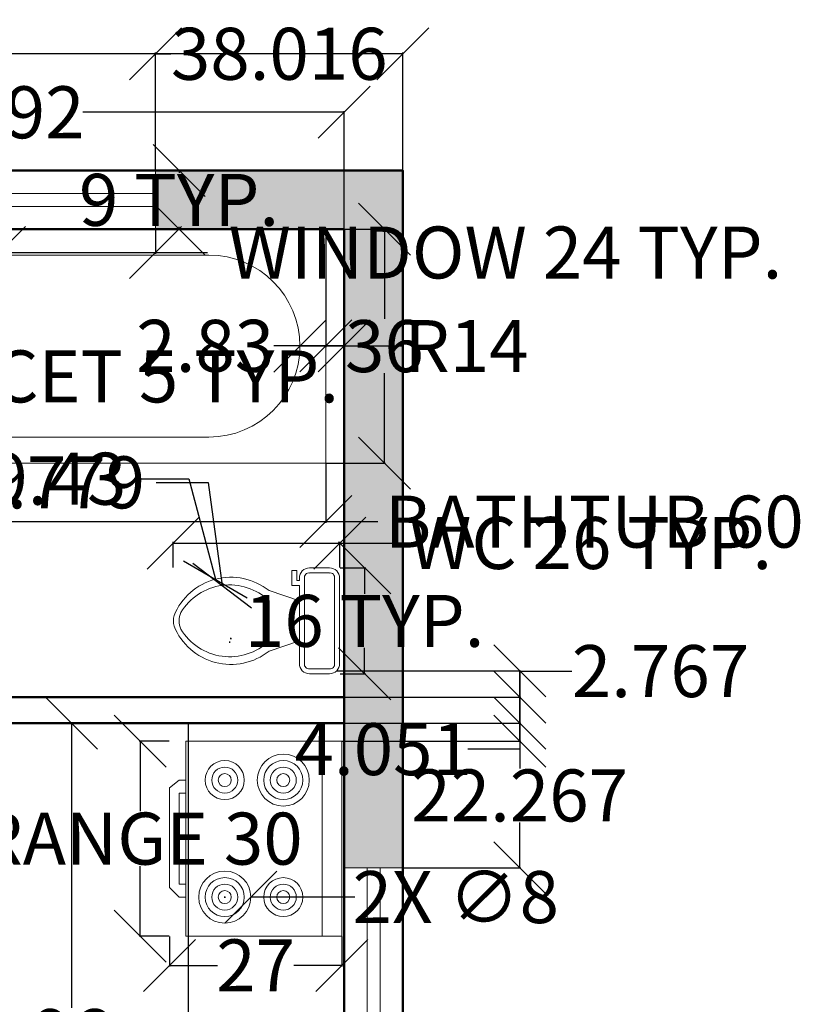
# Model space of a CAD drawing. Units: inches. Extents: x -87 to 308, y -349 to 42.
# Tile 6 of 6: x 188 to 308, y -110 to 42. Entities that reach past the tile are written whole.
import ezdxf

# ---------------------------------------------------------------- set-up
doc = ezdxf.new("R2010")
doc.units = ezdxf.units.IN
doc.header["$MEASUREMENT"] = 0
for name, color, linetype, lineweight in [('A-ANNO-DIMS', 2, 'Continuous', 18), ('A-EQPM', 8, 'Continuous', 20), ('A-FLOR-CASE', 9, 'Continuous', 25), ('A-FLOR-FIXT', 9, 'Continuous', 18), ('A-GLAZ', 4, 'Continuous', 18), ('A-WALL', 7, 'Continuous', 50), ('A-WALL-PATT', 251, 'Continuous', 13)]:
    doc.layers.add(name, color=color, linetype=linetype, lineweight=lineweight)
doc.styles.get("Standard").update_dxf_attribs({"font": 'arial.ttf'})
doc.dimstyles.get("Standard").update_dxf_attribs({"dimtxt": 8, "dimasz": 8, "dimexe": 0.18, "dimexo": 0.0625, "dimgap": 0.09, "dimtad": 0, "dimtih": 1, "dimtoh": 1, "dimdec": 0, "dimzin": 0, "dimdsep": 46, "dimlunit": 4, "dimtxsty": 'Standard', "dimblk": 'OBLIQUE', "dimcen": 0.09, "dimadec": 0, "dimazin": 0, "dimtfac": 1, "dimtdec": 0, "dimtofl": 0, "dimtmove": 0, "dimatfit": 3, "dimldrblk": 'OBLIQUE', "dimfxl": 1, "dimtolj": 1, "dimtzin": 0, "dimarcsym": 0})

# ---------------------------------------------------------------- blocks, each defined once
blk = doc.blocks.new('Toilet - top')
for p, q in [((9.5, -6), (9.5, -2)), ((-10, -8.5), (-8, -8.5)), ((-10, -9.5), (-10, -8.5)), ((-7, -9.5), (-10, -9.5)), ((-8, -8.5), (-8, -8)), ((-7, -8), (-7, -9.5)), ((-4, -8), (-6, -14)), ((4, -8), (6, -14)), ((4, -14), (-4, -14))]:
    blk.add_line(p, q)
blk.add_lwpolyline([(-7, -8), (8.5, -8, 0.414214), (10.5, -6), (10.5, -2, 0.414214), (8.5, 0), (-8.5, 0, 0.414214), (-10.5, -2), (-10.5, -6, 0.414214), (-8.5, -8), (-8, -8)], format="xyb")
for points in [[(8.5, -1), (-8.5, -1)], [(-9.5, -2), (-9.5, -6)], [(-8.5, -7), (8.5, -7)]]:
    blk.add_lwpolyline(points)
for centre, radius, start, end in [((-8.62, -1.88), 0.884, 81.8699, 188.1301), ((8.62, -1.88), 0.884, 351.8699, 98.1301), ((-8.62, -6.12), 0.884, 171.8699, 278.1301), ((8.62, -6.12), 0.884, 261.8699, 8.1301), ((3.52, -21.58), 12.17, 141.4691, 247.9714), ((4.2, -21.82), 11.33, 136.3677, 238.9468), ((-3.52, -21.58), 12.17, 292.0284, 38.5307), ((-4.2, -21.82), 11.33, 301.053, 43.6321), ((0, -27.88), 4, 245.7318, 294.2682), ((0, -29), 4, 254.8605, 285.1395)]:
    blk.add_arc(centre, radius, start, end)
blk = doc.blocks.new('Range-Oven - 30 in top')
for p, q in [((0, -3), (30, -3)), ((6, -24), (6, -25)), ((8, -25), (8, -24)), ((8, -24), (22, -24)), ((22, -25), (22, -24)), ((24, -24), (24, -25)), ((6, -25), (7.2, -26.5)), ((24, -25), (22.5, -26.5))]:
    blk.add_line(p, q)
for points in [[(8, -24), (0, -24), (0, 0), (30, 0), (30, -24), (22, -24)], [(8, -25), (22, -25)], [(22.5, -26.5), (7.2, -26.5)]]:
    blk.add_lwpolyline(points)
for centre, radius in [((6, -9), 4), ((6, -9), 3), ((24, -9), 3), ((6, -9), 2), ((24, -9), 2), ((6, -9), 1), ((24, -9), 1), ((6, -18), 3), ((24, -18), 4), ((24, -18), 3), ((6, -18), 2), ((24, -18), 2), ((6, -18), 1), ((24, -18), 1)]:
    blk.add_circle(centre, radius)
blk = doc.blocks.new('Bath Tub - 26 x 60 in.')
for p, q in [((8, -18), (10, -18)), ((9, -17), (9, -19))]:
    blk.add_line(p, q)
blk.add_lwpolyline([(0, -36), (0, 0), (60, 0), (60, -36)], close=True)
for points in [[(6, -4), (42, -4)], [(4, -30), (4, -6)], [(42, -32), (6, -32)]]:
    blk.add_lwpolyline(points)
for radius in [1.5, 1]:
    blk.add_circle((9, -18), radius)
for centre, radius, start, end in [((5.75, -5.75), 1.77, 81.8699, 188.1301), ((42, -18), 14, 270, 90), ((5.75, -30.25), 1.77, 171.8699, 278.1301)]:
    blk.add_arc(centre, radius, start, end)
blk = doc.blocks.new('WIN-48IN')
for p, q in [((0, 5.5), (48, 5.5)), ((0, 3.5), (48, 3.5))]:
    blk.add_line(p, q)
for points in [[(0, 0), (0, 9)], [(48, 9), (48, 0)]]:
    blk.add_lwpolyline(points)
blk = doc.blocks.new('WIN-24IN')
for p, q in [((0, 5.5), (24, 5.5)), ((0, 3.5), (24, 3.5))]:
    blk.add_line(p, q)
for points in [[(0, 0), (0, 9)], [(24, 9), (24, 0)]]:
    blk.add_lwpolyline(points)
blk = doc.blocks.new('_Oblique')
at = {"color": 0, "linetype": 'ByBlock', "lineweight": -2}
blk.add_line((-0.5, -0.5), (0.5, 0.5), dxfattribs=at)
blk = doc.blocks.new('*D25')
at = {"layer": 'A-ANNO-DIMS', "color": 0, "lineweight": -2, "transparency": 16777216}
for p, q in [((184.75, 9.27), (184.75, 5.55)), ((208.75, 9.27), (208.75, 5.55)), ((184.75, 5.73), (208.75, 5.73)), ((208.75, 5.73), (216.75, 5.73))]:
    blk.add_line(p, q, dxfattribs=at)
at = {"layer": 'Defpoints', "color": 0, "transparency": 16777216}
for p in [(184.75, 9.33), (208.75, 9.33), (208.75, 5.73)]:
    blk.add_point(p, dxfattribs=at)
at = {"layer": 'A-ANNO-DIMS', "color": 0, "lineweight": -2, "transparency": 16777216, "xscale": 8, "yscale": 8, "zscale": 8, "rotation": 180}
blk.add_blockref('_Oblique', (184.75, 5.73), dxfattribs=at)
at = {"layer": 'A-ANNO-DIMS', "color": 0, "lineweight": -2, "transparency": 16777216, "xscale": 8, "yscale": 8, "zscale": 8}
blk.add_blockref('_Oblique', (208.75, 5.73), dxfattribs=at)
at = {"layer": 'A-ANNO-DIMS', "color": 0, "transparency": 16777216, "insert": (262.54, 5.73), "char_height": 8, "attachment_point": 5}
blk.add_mtext('\\A1;WINDOW 24 TYP.', dxfattribs=at)
blk = doc.blocks.new('*D26')
at = {"layer": 'A-ANNO-DIMS', "color": 0, "lineweight": -2, "transparency": 16777216}
for p, q in [((208.81, 18.33), (212.53, 18.33)), ((212.35, 18.33), (212.35, 18.01)), ((208.81, 9.33), (212.53, 9.33)), ((212.35, 9.33), (212.35, 9.66))]:
    blk.add_line(p, q, dxfattribs=at)
at = {"layer": 'Defpoints', "color": 0, "transparency": 16777216}
for p in [(208.75, 18.33), (212.35, 18.33), (208.75, 9.33)]:
    blk.add_point(p, dxfattribs=at)
at = {"layer": 'A-ANNO-DIMS', "color": 0, "lineweight": -2, "transparency": 16777216, "xscale": 8, "yscale": 8, "zscale": 8}
for p, rotation in [((212.35, 18.33), 90), ((212.35, 9.33), 270)]:
    blk.add_blockref('_Oblique', p, dxfattribs=dict(at, rotation=rotation))
at = {"layer": 'A-ANNO-DIMS', "color": 0, "transparency": 16777216, "insert": (212.35, 13.83), "char_height": 8, "attachment_point": 5}
blk.add_mtext('\\A1;9 TYP.', dxfattribs=at)
blk = doc.blocks.new('*D27')
at = {"layer": 'A-ANNO-DIMS', "color": 0, "lineweight": -2, "transparency": 16777216}
for p, q in [((211.44, -42.74), (211.44, -38.78)), ((211.44, -38.96), (237.05, -38.96)), ((237.05, -42.74), (237.05, -38.78)), ((237.05, -38.96), (245.05, -38.96))]:
    blk.add_line(p, q, dxfattribs=at)
at = {"layer": 'Defpoints', "color": 0, "transparency": 16777216}
for p in [(237.05, -38.96), (211.44, -42.8), (237.05, -42.8)]:
    blk.add_point(p, dxfattribs=at)
at = {"layer": 'A-ANNO-DIMS', "color": 0, "lineweight": -2, "transparency": 16777216, "xscale": 8, "yscale": 8, "zscale": 8, "rotation": 180}
blk.add_blockref('_Oblique', (211.44, -38.96), dxfattribs=at)
at = {"layer": 'A-ANNO-DIMS', "color": 0, "lineweight": -2, "transparency": 16777216, "xscale": 8, "yscale": 8, "zscale": 8}
blk.add_blockref('_Oblique', (237.05, -38.96), dxfattribs=at)
at = {"layer": 'A-ANNO-DIMS', "color": 0, "transparency": 16777216, "insert": (275.63, -38.96), "char_height": 8, "attachment_point": 5}
blk.add_mtext('\\A1;WC 26 TYP.', dxfattribs=at)
blk = doc.blocks.new('*D28')
at = {"layer": 'A-ANNO-DIMS', "color": 0, "lineweight": -2, "transparency": 16777216}
for p, q in [((237.11, -42.8), (241.07, -42.8)), ((240.89, -42.8), (240.89, -46.76)), ((240.89, -59.07), (240.89, -55.11)), ((237.11, -59.07), (241.07, -59.07))]:
    blk.add_line(p, q, dxfattribs=at)
at = {"layer": 'Defpoints', "color": 0, "transparency": 16777216}
for p in [(237.05, -42.8), (237.05, -59.07), (240.89, -59.07)]:
    blk.add_point(p, dxfattribs=at)
at = {"layer": 'A-ANNO-DIMS', "color": 0, "lineweight": -2, "transparency": 16777216, "xscale": 8, "yscale": 8, "zscale": 8}
for p, rotation in [((240.89, -42.8), 90), ((240.89, -59.07), 270)]:
    blk.add_blockref('_Oblique', p, dxfattribs=dict(at, rotation=rotation))
at = {"layer": 'A-ANNO-DIMS', "color": 0, "transparency": 16777216, "insert": (240.89, -50.94), "char_height": 8, "attachment_point": 5}
blk.add_mtext('\\A1;16 TYP.', dxfattribs=at)
blk = doc.blocks.new('*D31')
at = {"layer": 'A-ANNO-DIMS', "color": 0, "lineweight": -2, "transparency": 16777216}
for p, q in [((151.98, -21.33), (151.98, -13.33)), ((151.98, -13.33), (159.98, -13.33)), ((151.29, -21.33), (152.16, -21.33)), ((151.98, -26.36), (151.98, -21.33)), ((151.29, -26.36), (152.16, -26.36))]:
    blk.add_line(p, q, dxfattribs=at)
at = {"layer": 'Defpoints', "color": 0, "transparency": 16777216}
for p in [(151.23, -21.33), (151.98, -21.33), (151.23, -26.36)]:
    blk.add_point(p, dxfattribs=at)
at = {"layer": 'A-ANNO-DIMS', "color": 0, "lineweight": -2, "transparency": 16777216, "xscale": 8, "yscale": 8, "zscale": 8}
for p, rotation in [((151.98, -21.33), 90), ((151.98, -26.36), 270)]:
    blk.add_blockref('_Oblique', p, dxfattribs=dict(at, rotation=rotation))
at = {"layer": 'A-ANNO-DIMS', "color": 0, "transparency": 16777216, "insert": (200.11, -13.33), "char_height": 8, "attachment_point": 5}
blk.add_mtext('\\A1;FAUCET 5 TYP.', dxfattribs=at)
blk = doc.blocks.new('*D41')
at = {"layer": 'A-ANNO-DIMS', "color": 0, "lineweight": -2, "transparency": 16777216}
for p, q in [((210.82, -69.44), (206.2, -69.44)), ((206.38, -69.44), (206.38, -80.21)), ((206.38, -99.44), (206.38, -88.66)), ((210.82, -99.44), (206.2, -99.44))]:
    blk.add_line(p, q, dxfattribs=at)
at = {"layer": 'Defpoints', "color": 0, "transparency": 16777216}
for p in [(210.88, -69.44), (206.38, -99.44), (210.88, -99.44)]:
    blk.add_point(p, dxfattribs=at)
at = {"layer": 'A-ANNO-DIMS', "color": 0, "lineweight": -2, "transparency": 16777216, "xscale": 8, "yscale": 8, "zscale": 8}
for p, rotation in [((206.38, -69.44), 90), ((206.38, -99.44), 270)]:
    blk.add_blockref('_Oblique', p, dxfattribs=dict(at, rotation=rotation))
at = {"layer": 'A-ANNO-DIMS', "color": 0, "transparency": 16777216, "insert": (206.38, -84.44), "char_height": 8, "attachment_point": 5}
blk.add_mtext('\\A1;RANGE 30', dxfattribs=at)
blk = doc.blocks.new('*D42')
at = {"layer": 'A-ANNO-DIMS', "color": 0, "lineweight": -2, "transparency": 16777216}
for p, q in [((210.88, -99.5), (210.88, -104.12)), ((237.38, -99.5), (237.38, -104.12)), ((210.88, -103.94), (218.24, -103.94)), ((237.38, -103.94), (230.02, -103.94))]:
    blk.add_line(p, q, dxfattribs=at)
at = {"layer": 'Defpoints', "color": 0, "transparency": 16777216}
for p in [(210.88, -99.44), (237.38, -99.44), (237.38, -103.94)]:
    blk.add_point(p, dxfattribs=at)
at = {"layer": 'A-ANNO-DIMS', "color": 0, "lineweight": -2, "transparency": 16777216, "xscale": 8, "yscale": 8, "zscale": 8, "rotation": 180}
blk.add_blockref('_Oblique', (210.88, -103.94), dxfattribs=at)
at = {"layer": 'A-ANNO-DIMS', "color": 0, "lineweight": -2, "transparency": 16777216, "xscale": 8, "yscale": 8, "zscale": 8}
blk.add_blockref('_Oblique', (237.38, -103.94), dxfattribs=at)
at = {"layer": 'A-ANNO-DIMS', "color": 0, "transparency": 16777216, "insert": (224.13, -103.94), "char_height": 8, "attachment_point": 5}
blk.add_mtext('\\A1;27', dxfattribs=at)
blk = doc.blocks.new('*D45')
at = {"layer": 'A-ANNO-DIMS', "color": 0, "lineweight": -2, "transparency": 16777216}
for p, q in [((174.93, -26.73), (174.93, -35.85)), ((234.93, -26.73), (234.93, -35.85)), ((174.93, -35.67), (234.93, -35.67)), ((234.93, -35.67), (242.93, -35.67))]:
    blk.add_line(p, q, dxfattribs=at)
at = {"layer": 'Defpoints', "color": 0, "transparency": 16777216}
for p in [(174.93, -26.67), (234.93, -26.67), (234.93, -35.67)]:
    blk.add_point(p, dxfattribs=at)
at = {"layer": 'A-ANNO-DIMS', "color": 0, "lineweight": -2, "transparency": 16777216, "xscale": 8, "yscale": 8, "zscale": 8, "rotation": 180}
blk.add_blockref('_Oblique', (174.93, -35.67), dxfattribs=at)
at = {"layer": 'A-ANNO-DIMS', "color": 0, "lineweight": -2, "transparency": 16777216, "xscale": 8, "yscale": 8, "zscale": 8}
blk.add_blockref('_Oblique', (234.93, -35.67), dxfattribs=at)
at = {"layer": 'A-ANNO-DIMS', "color": 0, "transparency": 16777216, "insert": (276.19, -35.67), "char_height": 8, "attachment_point": 5}
blk.add_mtext('\\A1;BATHTUB 60', dxfattribs=at)
blk = doc.blocks.new('*D46')
at = {"layer": 'A-ANNO-DIMS', "color": 0, "lineweight": -2, "transparency": 16777216}
for p, q in [((234.99, 9.33), (244.11, 9.33)), ((243.93, 9.33), (243.93, -4.49)), ((243.93, -26.67), (243.93, -12.85)), ((234.99, -26.67), (244.11, -26.67))]:
    blk.add_line(p, q, dxfattribs=at)
at = {"layer": 'Defpoints', "color": 0, "transparency": 16777216}
for p in [(234.93, 9.33), (243.93, 9.33), (234.93, -26.67)]:
    blk.add_point(p, dxfattribs=at)
at = {"layer": 'A-ANNO-DIMS', "color": 0, "lineweight": -2, "transparency": 16777216, "xscale": 8, "yscale": 8, "zscale": 8}
for p, rotation in [((243.93, 9.33), 90), ((243.93, -26.67), 270)]:
    blk.add_blockref('_Oblique', p, dxfattribs=dict(at, rotation=rotation))
at = {"layer": 'A-ANNO-DIMS', "color": 0, "transparency": 16777216, "insert": (243.93, -8.67), "char_height": 8, "attachment_point": 5}
blk.add_mtext('\\A1;36', dxfattribs=at)
blk = doc.blocks.new('*D47')
at = {"layer": 'A-ANNO-DIMS', "color": 0, "lineweight": -2, "transparency": 16777216}
for p, q in [((12.76, 18.39), (12.76, 36.48)), ((246.76, 18.39), (246.76, 36.48)), ((12.76, 36.3), (120.78, 36.3)), ((246.76, 36.3), (138.74, 36.3))]:
    blk.add_line(p, q, dxfattribs=at)
at = {"layer": 'Defpoints', "color": 0, "transparency": 16777216}
for p in [(246.76, 36.3), (12.76, 18.33), (246.76, 18.33)]:
    blk.add_point(p, dxfattribs=at)
at = {"layer": 'A-ANNO-DIMS', "color": 0, "lineweight": -2, "transparency": 16777216, "xscale": 8, "yscale": 8, "zscale": 8, "rotation": 180}
blk.add_blockref('_Oblique', (12.76, 36.3), dxfattribs=at)
at = {"layer": 'A-ANNO-DIMS', "color": 0, "lineweight": -2, "transparency": 16777216, "xscale": 8, "yscale": 8, "zscale": 8}
blk.add_blockref('_Oblique', (246.76, 36.3), dxfattribs=at)
at = {"layer": 'A-ANNO-DIMS', "color": 0, "transparency": 16777216, "insert": (129.76, 36.3), "char_height": 8, "attachment_point": 5}
blk.add_mtext('\\A1;234', dxfattribs=at)
blk = doc.blocks.new('*D50')
at = {"layer": 'A-ANNO-DIMS', "color": 0, "lineweight": -2, "transparency": 16777216}
for p, q in [((208.75, 18.39), (208.75, 36.48)), ((246.76, 18.39), (246.76, 36.48)), ((208.75, 36.3), (211.07, 36.3)), ((246.76, 36.3), (244.45, 36.3))]:
    blk.add_line(p, q, dxfattribs=at)
at = {"layer": 'Defpoints', "color": 0, "transparency": 16777216}
for p in [(246.76, 36.3), (208.75, 18.33), (246.76, 18.33)]:
    blk.add_point(p, dxfattribs=at)
at = {"layer": 'A-ANNO-DIMS', "color": 0, "lineweight": -2, "transparency": 16777216, "xscale": 8, "yscale": 8, "zscale": 8, "rotation": 180}
blk.add_blockref('_Oblique', (208.75, 36.3), dxfattribs=at)
at = {"layer": 'A-ANNO-DIMS', "color": 0, "lineweight": -2, "transparency": 16777216, "xscale": 8, "yscale": 8, "zscale": 8}
blk.add_blockref('_Oblique', (246.76, 36.3), dxfattribs=at)
at = {"layer": 'A-ANNO-DIMS', "color": 0, "transparency": 16777216, "insert": (227.76, 36.3), "char_height": 8, "attachment_point": 5}
blk.add_mtext('\\A1;38.016', dxfattribs=at)
blk = doc.blocks.new('*D57')
at = {"layer": 'A-ANNO-DIMS', "color": 0, "lineweight": -2, "transparency": 16777216}
for p, q in [((237.83, -66.67), (264.91, -66.67)), ((264.73, -66.67), (264.73, -73.63)), ((264.73, -88.94), (264.73, -81.98)), ((246.83, -88.94), (264.91, -88.94))]:
    blk.add_line(p, q, dxfattribs=at)
at = {"layer": 'Defpoints', "color": 0, "transparency": 16777216}
for p in [(237.76, -66.67), (246.76, -88.94), (264.73, -88.94)]:
    blk.add_point(p, dxfattribs=at)
at = {"layer": 'A-ANNO-DIMS', "color": 0, "lineweight": -2, "transparency": 16777216, "xscale": 8, "yscale": 8, "zscale": 8}
for p, rotation in [((264.73, -66.67), 90), ((264.73, -88.94), 270)]:
    blk.add_blockref('_Oblique', p, dxfattribs=dict(at, rotation=rotation))
at = {"layer": 'A-ANNO-DIMS', "color": 0, "transparency": 16777216, "insert": (264.73, -77.8), "char_height": 8, "attachment_point": 5}
blk.add_mtext('\\A1;22.267', dxfattribs=at)
blk = doc.blocks.new('*D61')
at = {"layer": 'A-ANNO-DIMS', "color": 0, "lineweight": -2, "transparency": 16777216}
for p, q in [((145.76, 9.39), (145.76, 27.48)), ((145.76, 27.3), (185.98, 27.3)), ((237.76, 27.3), (197.54, 27.3)), ((237.76, 9.39), (237.76, 27.48))]:
    blk.add_line(p, q, dxfattribs=at)
at = {"layer": 'Defpoints', "color": 0, "transparency": 16777216}
for p in [(237.76, 27.3), (145.76, 9.33), (237.76, 9.33)]:
    blk.add_point(p, dxfattribs=at)
at = {"layer": 'A-ANNO-DIMS', "color": 0, "lineweight": -2, "transparency": 16777216, "xscale": 8, "yscale": 8, "zscale": 8, "rotation": 180}
blk.add_blockref('_Oblique', (145.76, 27.3), dxfattribs=at)
at = {"layer": 'A-ANNO-DIMS', "color": 0, "lineweight": -2, "transparency": 16777216, "xscale": 8, "yscale": 8, "zscale": 8}
blk.add_blockref('_Oblique', (237.76, 27.3), dxfattribs=at)
at = {"layer": 'A-ANNO-DIMS', "color": 0, "transparency": 16777216, "insert": (191.76, 27.3), "char_height": 8, "attachment_point": 5}
blk.add_mtext('\\A1;92', dxfattribs=at)
blk = doc.blocks.new('*D74')
at = {"layer": 'A-ANNO-DIMS', "color": 0, "lineweight": -2, "transparency": 16777216}
for p, q in [((213.7, -66.67), (195.62, -66.67)), ((195.8, -66.67), (195.8, -110.49)), ((195.8, -162.67), (195.8, -118.84)), ((213.7, -162.67), (195.62, -162.67))]:
    blk.add_line(p, q, dxfattribs=at)
at = {"layer": 'Defpoints', "color": 0, "transparency": 16777216}
for p in [(195.8, -66.67), (213.76, -66.67), (213.76, -162.67)]:
    blk.add_point(p, dxfattribs=at)
at = {"layer": 'A-ANNO-DIMS', "color": 0, "lineweight": -2, "transparency": 16777216, "xscale": 8, "yscale": 8, "zscale": 8}
for p, rotation in [((195.8, -66.67), 90), ((195.8, -162.67), 270)]:
    blk.add_blockref('_Oblique', p, dxfattribs=dict(at, rotation=rotation))
at = {"layer": 'A-ANNO-DIMS', "color": 0, "transparency": 16777216, "insert": (195.8, -114.67), "char_height": 8, "attachment_point": 5}
blk.add_mtext('\\A1;96', dxfattribs=at)
blk = doc.blocks.new('*D85')
at = {"layer": 'A-ANNO-DIMS', "color": 0, "lineweight": -2, "transparency": 16777216}
for p, q in [((234.93, 9.27), (234.93, -8.81)), ((237.76, 9.27), (237.76, -8.81)), ((234.93, -8.63), (226.93, -8.63)), ((237.76, -8.63), (234.93, -8.63))]:
    blk.add_line(p, q, dxfattribs=at)
at = {"layer": 'Defpoints', "color": 0, "transparency": 16777216}
for p in [(234.93, 9.33), (237.76, 9.33), (234.93, -8.63)]:
    blk.add_point(p, dxfattribs=at)
at = {"layer": 'A-ANNO-DIMS', "color": 0, "lineweight": -2, "transparency": 16777216, "xscale": 8, "yscale": 8, "zscale": 8}
for p, rotation in [((234.93, -8.63), 179.9999999999999), ((237.76, -8.63), 359.9999999999999)]:
    blk.add_blockref('_Oblique', p, dxfattribs=dict(at, rotation=rotation))
at = {"layer": 'A-ANNO-DIMS', "color": 0, "transparency": 16777216, "insert": (216.38, -8.63), "char_height": 8, "attachment_point": 5}
blk.add_mtext('\\A1;2.83', dxfattribs=at)
blk = doc.blocks.new('*D87')
at = {"layer": 'A-ANNO-DIMS', "color": 0, "lineweight": -2, "transparency": 16777216}
for p, q in [((236.65, -58.62), (264.91, -58.62)), ((264.73, -58.62), (264.73, -62.67)), ((237.83, -62.67), (264.91, -62.67)), ((264.73, -62.67), (264.73, -70.67)), ((264.73, -70.67), (256.73, -70.67))]:
    blk.add_line(p, q, dxfattribs=at)
at = {"layer": 'Defpoints', "color": 0, "transparency": 16777216}
for p in [(236.59, -58.62), (237.76, -62.67), (264.73, -62.67)]:
    blk.add_point(p, dxfattribs=at)
at = {"layer": 'A-ANNO-DIMS', "color": 0, "lineweight": -2, "transparency": 16777216, "xscale": 8, "yscale": 8, "zscale": 8}
for p, rotation in [((264.73, -58.62), 90), ((264.73, -62.67), 270)]:
    blk.add_blockref('_Oblique', p, dxfattribs=dict(at, rotation=rotation))
at = {"layer": 'A-ANNO-DIMS', "color": 0, "transparency": 16777216, "insert": (243.75, -70.67), "char_height": 8, "attachment_point": 5}
blk.add_mtext('\\A1;4.051', dxfattribs=at)
blk = doc.blocks.new('*D88')
at = {"layer": 'A-ANNO-DIMS', "color": 0, "lineweight": -2, "transparency": 16777216}
for p, q in [((264.73, -66.67), (264.73, -58.67)), ((264.73, -58.67), (272.73, -58.67)), ((237.83, -66.67), (264.91, -66.67)), ((264.73, -69.44), (264.73, -66.67)), ((237.44, -69.44), (264.91, -69.44))]:
    blk.add_line(p, q, dxfattribs=at)
at = {"layer": 'Defpoints', "color": 0, "transparency": 16777216}
for p in [(237.76, -66.67), (264.73, -66.67), (237.38, -69.44)]:
    blk.add_point(p, dxfattribs=at)
at = {"layer": 'A-ANNO-DIMS', "color": 0, "lineweight": -2, "transparency": 16777216, "xscale": 8, "yscale": 8, "zscale": 8}
for p, rotation in [((264.73, -66.67), 90), ((264.73, -69.44), 270)]:
    blk.add_blockref('_Oblique', p, dxfattribs=dict(at, rotation=rotation))
at = {"layer": 'A-ANNO-DIMS', "color": 0, "transparency": 16777216, "insert": (286.38, -58.67), "char_height": 8, "attachment_point": 5}
blk.add_mtext('\\A1;2.767', dxfattribs=at)
blk = doc.blocks.new('*D96')
at = {"layer": 'A-ANNO-DIMS', "color": 0, "lineweight": -2, "transparency": 16777216}
for p, q in [((216.84, -8.67), (217.02, -8.67)), ((216.93, -8.76), (216.93, -8.58)), ((246.93, -8.67), (230.93, -8.67))]:
    blk.add_line(p, q, dxfattribs=at)
at = {"layer": 'Defpoints', "color": 0, "transparency": 16777216}
for p in [(216.93, -8.67), (230.93, -8.67)]:
    blk.add_point(p, dxfattribs=at)
at = {"layer": 'A-ANNO-DIMS', "color": 0, "lineweight": -2, "transparency": 16777216, "xscale": 8, "yscale": 8, "zscale": 8, "rotation": 180.0001186841147}
blk.add_blockref('_Oblique', (230.93, -8.67), dxfattribs=at)
at = {"layer": 'A-ANNO-DIMS', "color": 0, "transparency": 16777216, "insert": (256.56, -8.67), "char_height": 8, "attachment_point": 5}
blk.add_mtext('\\A1;R14', dxfattribs=at)
blk = doc.blocks.new('*D97')
at = {"layer": 'A-ANNO-DIMS', "color": 0, "lineweight": -2, "transparency": 16777216}
for p, q in [((205.86, -29.07), (213.86, -29.07)), ((213.86, -29.07), (217.93, -44.54)), ((220.23, -53.66), (220.41, -53.66)), ((220.32, -53.75), (220.32, -53.57))]:
    blk.add_line(p, q, dxfattribs=at)
at = {"layer": 'Defpoints', "color": 0, "transparency": 16777216}
for p in [(217.93, -44.54), (220.32, -53.66)]:
    blk.add_point(p, dxfattribs=at)
at = {"layer": 'A-ANNO-DIMS', "color": 0, "lineweight": -2, "transparency": 16777216, "xscale": 8, "yscale": 8, "zscale": 8, "rotation": 284.7189306886209}
blk.add_blockref('_Oblique', (217.93, -44.54), dxfattribs=at)
at = {"layer": 'A-ANNO-DIMS', "color": 0, "transparency": 16777216, "insert": (182.8, -29.07), "char_height": 8, "attachment_point": 5}
blk.add_mtext('\\A1;4X R9.43', dxfattribs=at)
blk = doc.blocks.new('*D98')
at = {"layer": 'A-ANNO-DIMS', "color": 0, "lineweight": -2, "transparency": 16777216}
for p, q in [((208.84, -29.63), (216.84, -29.63)), ((216.84, -29.63), (218.97, -45.49)), ((220.05, -54.19), (220.23, -54.19)), ((220.14, -54.28), (220.14, -54.1))]:
    blk.add_line(p, q, dxfattribs=at)
at = {"layer": 'Defpoints', "color": 0, "transparency": 16777216}
for p in [(218.97, -45.49), (220.14, -54.19)]:
    blk.add_point(p, dxfattribs=at)
at = {"layer": 'A-ANNO-DIMS', "color": 0, "lineweight": -2, "transparency": 16777216, "xscale": 8, "yscale": 8, "zscale": 8, "rotation": 277.6544285297157}
blk.add_blockref('_Oblique', (218.97, -45.49), dxfattribs=at)
at = {"layer": 'A-ANNO-DIMS', "color": 0, "transparency": 16777216, "insert": (182.66, -29.63), "char_height": 8, "attachment_point": 5}
blk.add_mtext('\\A1;4X R8.779', dxfattribs=at)
blk = doc.blocks.new('*D99')
at = {"layer": 'A-ANNO-DIMS', "color": 0, "lineweight": -2, "transparency": 16777216}
for p, q in [((219.29, -93.44), (219.47, -93.44)), ((219.38, -93.53), (219.38, -93.35)), ((239.38, -93.43), (223.38, -93.44))]:
    blk.add_line(p, q, dxfattribs=at)
at = {"layer": 'Defpoints', "color": 0, "transparency": 16777216}
for p in [(215.38, -93.44), (223.38, -93.44)]:
    blk.add_point(p, dxfattribs=at)
at = {"layer": 'A-ANNO-DIMS', "color": 0, "lineweight": -2, "transparency": 16777216, "xscale": 8, "yscale": 8, "zscale": 8, "rotation": 180.0016615776052}
blk.add_blockref('_Oblique', (223.38, -93.44), dxfattribs=at)
at = {"layer": 'A-ANNO-DIMS', "color": 0, "transparency": 16777216, "insert": (254.9, -93.43), "char_height": 8, "attachment_point": 5}
blk.add_mtext('\\A1;2X ∅8', dxfattribs=at)

msp = doc.modelspace()

# ---------------------------------------------------------------- hatches: boundary and pattern name
at = {"layer": 'A-WALL-PATT'}
h = msp.add_hatch(color=256, dxfattribs=at)
h.dxf.hatch_style = 1
h.paths.add_polyline_path([(246.7637, 18.332), (208.748, 18.332), (208.748, 9.332), (234.9321, 9.332), (237.7637, 9.332), (237.7637, -88.9351), (246.7637, -88.9351)])

# ---------------------------------------------------------------- linework, layer by layer
at = {"layer": 'A-FLOR-CASE'}
msp.add_line((213.7637, -66.668), (213.7637, -162.668), dxfattribs=at)
at = {"layer": 'A-WALL'}
for p, q in [((145.7637, 9.332), (237.7637, 9.332)), ((237.7637, 9.332), (237.7637, -162.668)), ((181.7637, -62.668), (237.7637, -62.668)), ((181.7637, -66.668), (237.7637, -66.668))]:
    msp.add_line(p, q, dxfattribs=at)
msp.add_lwpolyline([(142.7127, -323.668), (12.7637, -323.668), (12.7637, 18.332), (246.7637, 18.332), (246.7637, -323.668), (172.7127, -323.668)], dxfattribs=at)

# ---------------------------------------------------------------- block references
at = {"layer": 'A-EQPM', "rotation": 270}
msp.add_blockref('Range-Oven - 30 in top', (237.3805, -69.4351), dxfattribs=at)
at = {"layer": 'A-FLOR-FIXT'}
msp.add_blockref('Bath Tub - 26 x 60 in.', (174.9321, 9.332), dxfattribs=at)
at = {"layer": 'A-FLOR-FIXT', "xscale": 0.7748713842371889, "yscale": 0.7748713842371889, "zscale": 0.7748713842371889, "rotation": 270}
msp.add_blockref('Toilet - top', (237.046, -50.9351), dxfattribs=at)
at = {"layer": 'A-GLAZ'}
msp.add_blockref('WIN-24IN', (184.748, 9.332), dxfattribs=at)
at = {"layer": 'A-GLAZ', "rotation": 270.0000000000002}
msp.add_blockref('WIN-48IN', (237.7637, -88.935), dxfattribs=at)

# ---------------------------------------------------------------- dimensions: what is measured, and where the dimension line sits
at = {"layer": 'A-ANNO-DIMS'}
for base, p1, p2, override, picture, middle in [((246.7637, 36.2965), (12.7637, 18.332), (246.7637, 18.332), {"dimdec": 0, "dimlfac": 1, "dimrnd": 0, "dimzin": 0, "dimdsep": 46, "dimlunit": 2}, '*D47', (129.7637, 36.2965)), ((246.7637, 36.2965), (208.748, 18.332), (246.7637, 18.332), {"dimdec": 3, "dimlfac": 1, "dimrnd": 0, "dimzin": 0, "dimdsep": 46, "dimlunit": 2}, '*D50', (227.7558, 36.2965)), ((237.7637, 27.2965), (145.7637, 9.332), (237.7637, 9.332), {"dimdec": 0, "dimlfac": 1, "dimrnd": 0, "dimzin": 0, "dimdsep": 46, "dimlunit": 2}, '*D61', (191.7637, 27.2965)), ((237.3804738019, -103.9351157857), (210.8804738019, -99.4351157857), (237.3804738019, -99.4351157857), {"dimdec": 0, "dimlfac": 1, "dimrnd": 0, "dimzin": 0, "dimdsep": 46, "dimlunit": 2}, '*D42', (224.1304738019, -103.9351157857))]:
    dim = msp.add_linear_dim(base=base, p1=p1, p2=p2, dimstyle='Standard', override=override, dxfattribs=at)
    dim.commit()
    dim.dimension.update_dxf_attribs({"geometry": picture, "text_midpoint": middle})
for base, p1, p2, angle, text, picture, middle in [((212.348, 18.332), (208.748, 9.332), (208.748, 18.332), 90, '<> TYP.', '*D26', (212.348, 13.832)), ((151.983, -21.3298), (151.2279, -26.3642), (151.2279, -21.3298), 90, 'FAUCET <> TYP.', '*D31', (200.114, -13.3298)), ((240.887, -59.0713), (237.046, -42.799), (237.046, -59.0713), 270, '<> TYP.', '*D28', (240.887, -50.9351)), ((206.3805, -99.4351), (210.8805, -69.4351), (210.8805, -99.4351), 270, 'RANGE <>', '*D41', (206.3805, -84.4351))]:
    dim = msp.add_linear_dim(base=base, p1=p1, p2=p2, angle=angle, text=text, dimstyle='Standard', override={"dimdec": 0, "dimlfac": 1, "dimrnd": 0, "dimzin": 0, "dimdsep": 46, "dimlunit": 2}, dxfattribs=at)
    dim.commit()
    dim.dimension.update_dxf_attribs({"geometry": picture, "text_midpoint": middle})
for base, p1, p2, text, picture, middle in [((208.748, 5.732), (184.748, 9.332), (208.748, 9.332), 'WINDOW <> TYP.', '*D25', (262.5433, 5.732)), ((237.046, -38.958), (211.4394, -42.799), (237.046, -42.799), 'WC <> TYP.', '*D27', (275.6326, -38.958)), ((234.9321, -35.668), (174.9321, -26.668), (234.9321, -26.668), 'BATHTUB <>', '*D45', (276.1926, -35.668))]:
    dim = msp.add_linear_dim(base=base, p1=p1, p2=p2, text=text, dimstyle='Standard', override={"dimdec": 0, "dimlfac": 1, "dimrnd": 0, "dimzin": 0, "dimdsep": 46, "dimlunit": 2}, dxfattribs=at)
    dim.commit()
    dim.dimension.update_dxf_attribs({"geometry": picture, "text_midpoint": middle})
for base, p1, p2, angle, override, picture, middle in [((243.9321, 9.332), (234.9321, -26.668), (234.9321, 9.332), 90, {"dimdec": 0, "dimlfac": 1, "dimrnd": 0, "dimzin": 0, "dimdsep": 46, "dimlunit": 2}, '*D46', (243.9321, -8.668)), ((234.9321, -8.6325), (237.7637, 9.332), (234.9321, 9.332), 180, {"dimdec": 2, "dimlfac": 1, "dimrnd": 0, "dimzin": 0, "dimdsep": 46, "dimlunit": 2}, '*D85', (216.3837, -8.6325)), ((264.7282, -66.668), (237.3805, -69.4351), (237.7637, -66.668), 90, {"dimdec": 3, "dimlfac": 1, "dimrnd": 0, "dimzin": 0, "dimdsep": 46, "dimlunit": 2}, '*D88', (286.3843, -58.668)), ((264.7282, -62.668), (236.5921, -58.6174), (237.7637, -62.668), 90, {"dimdec": 3, "dimlfac": 1, "dimrnd": 0, "dimzin": 0, "dimdsep": 46, "dimlunit": 2}, '*D87', (243.7514, -70.668)), ((195.7992, -66.668), (213.7637, -162.668), (213.7637, -66.668), 90, {"dimdec": 0, "dimlfac": 1, "dimrnd": 0, "dimzin": 0, "dimdsep": 46, "dimlunit": 2}, '*D74', (195.7992, -114.668)), ((264.7282, -88.9351), (237.7637, -66.668), (246.7637, -88.9351), 90, {"dimdec": 3, "dimlfac": 1, "dimrnd": 0, "dimzin": 0, "dimdsep": 46, "dimlunit": 2}, '*D57', (264.7282, -77.8016))]:
    dim = msp.add_linear_dim(base=base, p1=p1, p2=p2, angle=angle, dimstyle='Standard', override=override, dxfattribs=at)
    dim.commit()
    dim.dimension.update_dxf_attribs({"geometry": picture, "text_midpoint": middle})
dim = msp.add_radius_dim(center=(216.9321, -8.668), mpoint=(230.9321, -8.668), dimstyle='Standard', override={"dimdec": 0, "dimlfac": 1, "dimrnd": 0, "dimzin": 0, "dimdsep": 46, "dimlunit": 2}, dxfattribs=at)
dim.commit()
dim.dimension.update_dxf_attribs({"geometry": '*D96', "text_midpoint": (256.5637, -8.668)})
for center, mpoint, override, picture, middle in [((220.1403, -54.1895), (218.971, -45.4891), {"dimdec": 3, "dimlfac": 1, "dimrnd": 0, "dimzin": 0, "dimdsep": 46, "dimlunit": 2}, '*D98', (182.6598, -29.6317)), ((220.3239, -53.6623), (217.9281, -44.5423), {"dimdec": 2, "dimlfac": 1, "dimrnd": 0, "dimzin": 0, "dimdsep": 46, "dimlunit": 2}, '*D97', (182.7988, -29.0674))]:
    dim = msp.add_radius_dim(center=center, mpoint=mpoint, text='4X <>', dimstyle='Standard', override=override, dxfattribs=at)
    dim.commit()
    dim.dimension.update_dxf_attribs({"geometry": picture, "text_midpoint": middle})
dim = msp.add_diameter_dim_2p(p1=(215.3805, -93.4352), p2=(223.3805, -93.435), text='2X <>', dimstyle='Standard', override={"dimdec": 0, "dimlfac": 1, "dimrnd": 0, "dimzin": 0, "dimdsep": 46, "dimlunit": 2}, dxfattribs=at)
dim.commit()
dim.dimension.update_dxf_attribs({"geometry": '*D99', "text_midpoint": (239.3805, -93.4345)})

doc.saveas('drawing.dxf')
